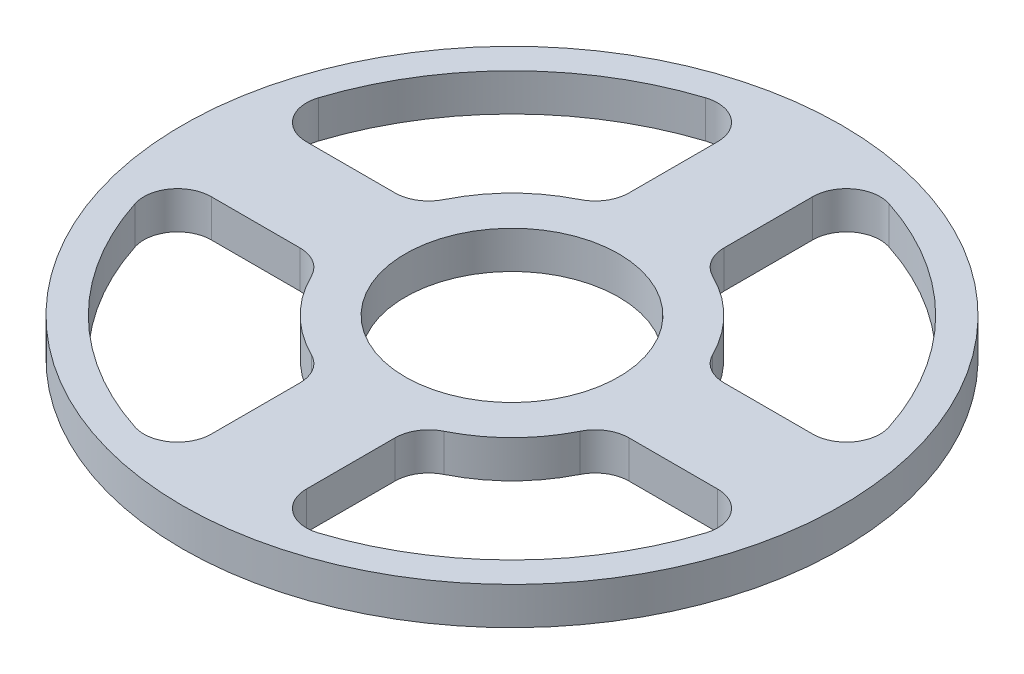
SolidWorks part; units mm, degrees
material "Plain Carbon Steel"
ref_plane "Front Plane" through (0, 0, 0) normal (0, 0, 1) x (1, 0, 0)
ref_plane "Top Plane" through (0, 0, 0) normal (0, 1, 0) x (1, 0, 0)
ref_plane "Right Plane" through (0, 0, 0) normal (1, 0, 0) x (0, 0, -1)
sketch "Web Disc Profile Ø90" plane through (0, 0, 0) normal (0, 1, 0) x (1, 0, 0)
  circle A0 centre (0, 0) radius 44
  dimension "D1" = 88
extrude "Web Disc Ø90x5" add sketch "Web Disc Profile Ø90" along normal blind 5
sketch "Bore and Spoke Windows Profile" plane through (0, 5, 0) normal (0, 1, 0) x (1, 0, 0)
  line L0 (6.35, 21.9665) -> (6.35, 33.8013)
  line L1 (6.35, -21.9665) -> (6.35, -33.8013)
  line L2 (21.9665, -6.35) -> (33.8013, -6.35)
  line L3 (-21.9665, -6.35) -> (-33.8013, -6.35)
  line L4 (6.35, 21.9665) -> (6.35, 33.8013)
  line L5 (21.9665, 6.35) -> (33.8013, 6.35)
  line L6 (-6.35, -21.9665) -> (-6.35, -33.8013)
  line L7 (-6.35, 21.9665) -> (-6.35, 33.8013)
  line L8 (-21.9665, 6.35) -> (-33.8013, 6.35)
  arc A0 (38.086, 12.2254) -> (12.2254, 38.086) centre (0, 0) ccw
  arc A1 (17.9318, 8.8571) -> (8.8571, 17.9318) centre (0, 0) ccw
  arc A2 (12.2254, 38.086) -> (6.35, 33.8013) centre (10.85, 33.8013) ccw
  arc A3 (6.35, 21.9665) -> (8.8571, 17.9318) centre (10.85, 21.9665) ccw
  arc A4 (17.9318, 8.8571) -> (21.9665, 6.35) centre (21.9665, 10.85) ccw
  arc A5 (33.8013, 6.35) -> (38.086, 12.2254) centre (33.8013, 10.85) ccw
  arc A6 (38.086, -12.2254) -> (33.8013, -6.35) centre (33.8013, -10.85) ccw
  arc A7 (12.2254, -38.086) -> (38.086, -12.2254) centre (0, 0) ccw
  arc A8 (6.35, -33.8013) -> (12.2254, -38.086) centre (10.85, -33.8013) ccw
  arc A9 (8.8571, -17.9318) -> (6.35, -21.9665) centre (10.85, -21.9665) ccw
  arc A10 (8.8571, -17.9318) -> (17.9318, -8.8571) centre (0, 0) ccw
  arc A11 (21.9665, -6.35) -> (17.9318, -8.8571) centre (21.9665, -10.85) ccw
  arc A12 (-12.2254, -38.086) -> (-6.35, -33.8013) centre (-10.85, -33.8013) ccw
  arc A13 (-38.086, -12.2254) -> (-12.2254, -38.086) centre (0, 0) ccw
  arc A14 (-33.8013, -6.35) -> (-38.086, -12.2254) centre (-33.8013, -10.85) ccw
  arc A15 (-17.9318, -8.8571) -> (-21.9665, -6.35) centre (-21.9665, -10.85) ccw
  arc A16 (-17.9318, -8.8571) -> (-8.8571, -17.9318) centre (0, 0) ccw
  arc A17 (-6.35, -21.9665) -> (-8.8571, -17.9318) centre (-10.85, -21.9665) ccw
  arc A18 (-38.086, 12.2254) -> (-33.8013, 6.35) centre (-33.8013, 10.85) ccw
  arc A19 (-12.2254, 38.086) -> (-38.086, 12.2254) centre (0, 0) ccw
  arc A20 (-6.35, 33.8013) -> (-12.2254, 38.086) centre (-10.85, 33.8013) ccw
  arc A21 (-8.8571, 17.9318) -> (-6.35, 21.9665) centre (-10.85, 21.9665) ccw
  arc A22 (-8.8571, 17.9318) -> (-17.9318, 8.8571) centre (0, 0) ccw
  arc A23 (-21.9665, 6.35) -> (-17.9318, 8.8571) centre (-21.9665, 10.85) ccw
  circle A24 centre (0, 0) radius 14.25
  point P3 (6.35, 0)
  point P4 (0, 50.4402)
  point P5 (6.35, 50.4402)
  point P6 (-6.35, 0)
  point P7 (-6.35, 50.4402)
  point P9 (6.35, 6.35)
  point P10 (56.5615, 0)
  point P12 (56.5615, 6.35)
  dimension "D1" = 80
  dimension "D4" = 40
  dimension "D3" = 28.5
  dimension "D5" = 4.5
  dimension "D8" = 4.5
  dimension "D9" = 4.5
  dimension "D10" = 4.5
  dimension "D6" = 33.8013
  dimension "D7" = 11.8348
  dimension "D11" = 10.85
  dimension "D12" = 11.8348
  dimension "D13" = 11.1165
  dimension "D14" = 6.35
  dimension "D2" = 4
extrude "Centre Bore and 4x Spoke Windows" cut sketch "Bore and Spoke Windows Profile" against normal blind 44 contours L8 A23 A22 A21 L7 A20 A19 A18 | L5 A5 A0 A2 L0 A3 A1 A4 | L2 A11 A10 A9 L1 A8 A7 A6 | L6 A17 A16 A15 L3 A14 A13 A12 | A24
